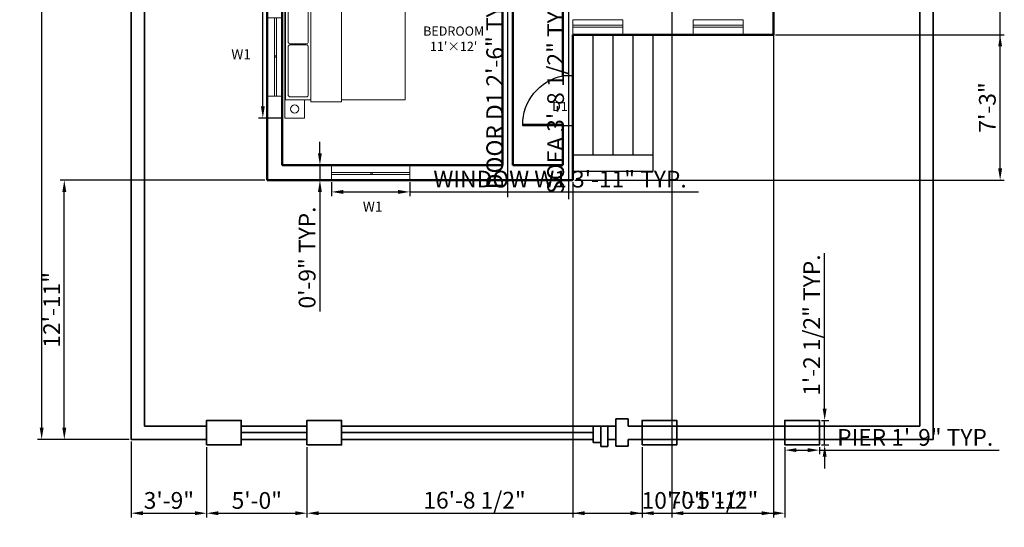
# Model space of a CAD drawing. Units: inches. Extents: x 452 to 1041, y 578 to 1412.
# Tile 1 of 3: x 452 to 1041, y 578 to 881. Entities that reach past the tile are written whole.
import ezdxf

# ---------------------------------------------------------------- set-up
doc = ezdxf.new("R2010")
doc.units = ezdxf.units.IN
doc.linetypes.add('ACAD_ISO03W100', pattern=[30, 12, -18])
doc.layers.get('Defpoints').update_dxf_attribs({"linetype": 'ACAD_ISO03W100'})
for name, color, linetype, lineweight in [('A-ANNO-DIMS', 2, 'Continuous', 18), ('A-ANNO-TEXT', 7, 'Continuous', 18), ('A-AREA-IDEN', 7, 'Continuous', 25), ('A-DOOR', 3, 'Continuous', 25), ('A-FLOR-STRS', 7, 'Continuous', 25), ('A-FURN', 8, 'Continuous', 18), ('A-GLAZ', 160, 'Continuous', 20), ('A-WALL', 7, 'Continuous', 50), ('C-PROP', 7, 'Continuous', 35)]:
    doc.layers.add(name, color=color, linetype=linetype, lineweight=lineweight)
doc.styles.get("Standard").update_dxf_attribs({"font": 'times.ttf'})
doc.dimstyles.new('ISO-25', dxfattribs={"dimscale": 2, "dimtxt": 5, "dimasz": 3.5, "dimexe": 1.25, "dimexo": 0.625, "dimtad": 1, "dimdsep": 46, "dimlunit": 3, "dimtxsty": 'Standard', "dimcen": 2.5, "dimadec": 0, "dimazin": 0, "dimtfac": 1, "dimtmove": 0, "dimatfit": 3, "dimfxl": 1, "dimarcsym": 0})

# ---------------------------------------------------------------- blocks, each defined once
blk = doc.blocks.new('D1')
for p, q in [((734.6, 1191.77), (733.6, 1191.77)), ((733.6, 1191.77), (733.6, 1167.77)), ((734.6, 1161.77), (734.6, 1191.77)), ((704.6, 1161.77), (704.6, 1167.77))]:
    blk.add_line(p, q)
blk.add_arc((733.85, 1161.94), 29.82, 89.51971, 168.74109)
blk = doc.blocks.new('W')
for p, q in [((913.24, 916.29), (913.24, 963.09)), ((913.24, 963.09), (922.24, 963.09)), ((917.74, 963.09), (917.74, 916.29)), ((918.94, 963.09), (918.94, 916.29)), ((922.24, 963.09), (922.24, 916.29)), ((917.74, 940.48), (918.94, 940.48)), ((917.74, 939.69), (918.94, 939.69)), ((922.24, 916.29), (913.24, 916.29))]:
    blk.add_line(p, q)
blk = doc.blocks.new('V')
for p, q in [((599.59, 961.66), (599.59, 991.66)), ((599.59, 991.66), (608.59, 991.66)), ((604.09, 961.66), (604.09, 991.66)), ((604.09, 991.66), (605.29, 991.66)), ((605.29, 991.66), (605.29, 961.66)), ((608.59, 991.66), (608.59, 961.66)), ((608.59, 961.66), (599.59, 961.66)), ((608.59, 961.66), (604.09, 961.66))]:
    blk.add_line(p, q)
blk = doc.blocks.new('*D8')
at = {"layer": 'A-ANNO-DIMS', "color": 0, "lineweight": -2, "transparency": 16777216}
for p, q in [((481.13, 1350.33), (462.24, 1350.33)), ((464.74, 1343.33), (464.74, 637.33)), ((481.13, 630.33), (462.24, 630.33))]:
    blk.add_line(p, q, dxfattribs=at)
at = {"layer": 'A-ANNO-DIMS', "color": 0, "lineweight": 70, "transparency": 16777216}
for points in [[(463.58, 1343.33), (465.91, 1343.33), (464.74, 1350.33)], [(463.58, 637.33), (465.91, 637.33), (464.74, 630.33)]]:
    blk.add_solid(points, dxfattribs=at)
at = {"layer": 'Defpoints', "color": 0, "lineweight": 70, "transparency": 16777216}
for p in [(482.38, 1350.33), (464.74, 630.33), (482.38, 630.33)]:
    blk.add_point(p, dxfattribs=at)
at = {"layer": 'A-ANNO-DIMS', "color": 0, "transparency": 16777216, "insert": (458.41, 990.33), "char_height": 10, "attachment_point": 5, "rotation": 90}
blk.add_mtext("60'", dxfattribs=at)
blk = doc.blocks.new('BED-FRAME-AND-SIDE-TABLES')
for p, q in [((0, 76.85), (15.53, 76.85)), ((0, 10.85), (0, 76.85)), ((0.5, 76.85), (0.5, 10.85)), ((33.97, 76.85), (72, 76.85)), ((72, 76.85), (72, 10.85)), ((15.53, 10.85), (0, 10.85)), ((72, 10.85), (33.97, 10.85))]:
    blk.add_line(p, q)
for points in [[(0, 76.85), (11.87, 76.85), (11.87, 87.71), (0, 87.71)], [(15.53, 78), (33.97, 78), (33.97, 9.68), (15.53, 9.68)], [(0, 0), (11.87, 0), (11.87, 10.85), (0, 10.85)]]:
    blk.add_lwpolyline(points, close=True)
for centre in [(5.89, 82.36), (5.89, 5.42)]:
    blk.add_circle(centre, 2.46)
blk = doc.blocks.new('BOUNDARY-PIER')
blk.add_lwpolyline([(0, 0), (20.76, 0), (20.76, 14.71), (0, 14.71)], close=True)
blk = doc.blocks.new('*D16')
at = {"layer": 'A-ANNO-DIMS', "color": 0, "lineweight": -2, "transparency": 16777216}
for p, q in [((638.26, 784.2), (638.26, 775.93)), ((685.06, 784.2), (685.06, 775.93)), ((645.26, 778.43), (678.06, 778.43)), ((685.06, 778.43), (857.83, 778.43))]:
    blk.add_line(p, q, dxfattribs=at)
at = {"layer": 'A-ANNO-DIMS', "color": 0, "lineweight": 70, "transparency": 16777216}
for points in [[(645.26, 779.6), (645.26, 777.26), (638.26, 778.43)], [(678.06, 779.6), (678.06, 777.26), (685.06, 778.43)]]:
    blk.add_solid(points, dxfattribs=at)
at = {"layer": 'Defpoints', "color": 0, "lineweight": 70, "transparency": 16777216}
for p in [(638.26, 785.45), (685.06, 785.45), (685.06, 778.43)]:
    blk.add_point(p, dxfattribs=at)
at = {"layer": 'A-ANNO-DIMS', "color": 0, "transparency": 16777216, "insert": (774.94, 784.79), "char_height": 10, "attachment_point": 5}
blk.add_mtext('WINDOW W1 3\'-11" TYP.', dxfattribs=at)
blk = doc.blocks.new('*D17')
at = {"layer": 'A-ANNO-DIMS', "color": 0, "lineweight": -2, "transparency": 16777216}
for p, q in [((631.24, 801.45), (631.24, 808.45)), ((637.01, 794.45), (628.74, 794.45)), ((631.24, 794.45), (631.24, 785.45)), ((637.01, 785.45), (628.74, 785.45)), ((631.24, 778.45), (631.24, 706.88))]:
    blk.add_line(p, q, dxfattribs=at)
at = {"layer": 'A-ANNO-DIMS', "color": 0, "lineweight": 70, "transparency": 16777216}
for points in [[(630.07, 801.45), (632.4, 801.45), (631.24, 794.45)], [(630.07, 778.45), (632.4, 778.45), (631.24, 785.45)]]:
    blk.add_solid(points, dxfattribs=at)
at = {"layer": 'Defpoints', "color": 0, "lineweight": 70, "transparency": 16777216}
for p in [(638.26, 794.45), (631.24, 785.45), (638.26, 785.45)]:
    blk.add_point(p, dxfattribs=at)
at = {"layer": 'A-ANNO-DIMS', "color": 0, "transparency": 16777216, "insert": (624.89, 739.17), "char_height": 10, "attachment_point": 5, "rotation": 90}
blk.add_mtext('0\'-9" TYP.', dxfattribs=at)
blk = doc.blocks.new('*D22')
at = {"layer": 'A-ANNO-DIMS', "color": 0, "lineweight": -2, "transparency": 16777216}
for p, q in [((740.23, 944.45), (746, 944.45)), ((743.5, 937.45), (743.5, 921.33)), ((740.23, 914.33), (746, 914.33)), ((743.5, 914.33), (743.5, 775.21))]:
    blk.add_line(p, q, dxfattribs=at)
at = {"layer": 'A-ANNO-DIMS', "color": 0, "lineweight": 70, "transparency": 16777216}
for points in [[(742.34, 937.45), (744.67, 937.45), (743.5, 944.45)], [(742.34, 921.33), (744.67, 921.33), (743.5, 914.33)]]:
    blk.add_solid(points, dxfattribs=at)
at = {"layer": 'Defpoints', "color": 0, "lineweight": 70, "transparency": 16777216}
for p in [(738.98, 944.45), (738.98, 914.33), (743.5, 914.33)]:
    blk.add_point(p, dxfattribs=at)
at = {"layer": 'A-ANNO-DIMS', "color": 0, "transparency": 16777216, "insert": (737.14, 841.27), "char_height": 10, "attachment_point": 5, "rotation": 90}
blk.add_mtext('DOOR D1 2\'-6" TYP.', dxfattribs=at)
blk = doc.blocks.new('*D26')
at = {"layer": 'A-ANNO-DIMS', "color": 0, "lineweight": -2, "transparency": 16777216}
for p, q in [((909.42, 625.82), (909.42, 621.45)), ((930.18, 625.82), (930.18, 621.45)), ((916.42, 623.95), (923.18, 623.95)), ((930.18, 623.95), (1037.72, 623.95))]:
    blk.add_line(p, q, dxfattribs=at)
at = {"layer": 'A-ANNO-DIMS', "color": 0, "lineweight": 70, "transparency": 16777216}
for points in [[(916.42, 625.12), (916.42, 622.79), (909.42, 623.95)], [(923.18, 625.12), (923.18, 622.79), (930.18, 623.95)]]:
    blk.add_solid(points, dxfattribs=at)
at = {"layer": 'Defpoints', "color": 0, "lineweight": 70, "transparency": 16777216}
for p in [(909.42, 627.07), (930.18, 627.07), (930.18, 623.95)]:
    blk.add_point(p, dxfattribs=at)
at = {"layer": 'A-ANNO-DIMS', "color": 0, "transparency": 16777216, "insert": (987.45, 630.3), "char_height": 10, "attachment_point": 5}
blk.add_mtext('PIER 1\'-9" TYP.', dxfattribs=at)
blk = doc.blocks.new('*D27')
at = {"layer": 'A-ANNO-DIMS', "color": 0, "lineweight": -2, "transparency": 16777216}
for p, q in [((933.29, 648.78), (933.29, 741.71)), ((931.43, 641.78), (935.79, 641.78)), ((933.29, 627.07), (933.29, 641.78)), ((931.43, 627.07), (935.79, 627.07)), ((933.29, 620.07), (933.29, 613.07))]:
    blk.add_line(p, q, dxfattribs=at)
at = {"layer": 'A-ANNO-DIMS', "color": 0, "lineweight": 70, "transparency": 16777216}
for points in [[(932.12, 648.78), (934.46, 648.78), (933.29, 641.78)], [(932.12, 620.07), (934.46, 620.07), (933.29, 627.07)]]:
    blk.add_solid(points, dxfattribs=at)
at = {"layer": 'Defpoints', "color": 0, "lineweight": 70, "transparency": 16777216}
for p in [(930.18, 641.78), (933.29, 641.78), (930.18, 627.07)]:
    blk.add_point(p, dxfattribs=at)
at = {"layer": 'A-ANNO-DIMS', "color": 0, "transparency": 16777216, "insert": (926.81, 698.75), "char_height": 10, "attachment_point": 5, "rotation": 90}
blk.add_mtext('1\'-2 1/2" TYP.', dxfattribs=at)
blk = doc.blocks.new('*D32')
at = {"layer": 'A-ANNO-DIMS', "color": 0, "lineweight": -2, "transparency": 16777216}
for p, q in [((785.53, 953.88), (777.57, 953.88)), ((780.07, 946.88), (780.07, 916.19)), ((785.53, 909.19), (777.57, 909.19)), ((780.07, 909.19), (780.07, 774.01))]:
    blk.add_line(p, q, dxfattribs=at)
at = {"layer": 'A-ANNO-DIMS', "color": 0, "lineweight": 70, "transparency": 16777216}
for points in [[(778.91, 946.88), (781.24, 946.88), (780.07, 953.88)], [(778.91, 916.19), (781.24, 916.19), (780.07, 909.19)]]:
    blk.add_solid(points, dxfattribs=at)
at = {"layer": 'Defpoints', "color": 0, "lineweight": 70, "transparency": 16777216}
for p in [(786.78, 953.88), (780.07, 909.19), (786.78, 909.19)]:
    blk.add_point(p, dxfattribs=at)
at = {"layer": 'A-ANNO-DIMS', "color": 0, "transparency": 16777216, "insert": (773.59, 838.1), "char_height": 10, "attachment_point": 5, "rotation": 90}
blk.add_mtext('SOFA 3\'-8 1/2" TYP.', dxfattribs=at)
blk = doc.blocks.new('*D34')
at = {"layer": 'A-ANNO-DIMS', "color": 0, "lineweight": -2, "transparency": 16777216}
for p, q in [((597.08, 910.3), (597.08, 1067.89)), ((608.99, 910.3), (594.58, 910.3)), ((597.08, 829.6), (597.08, 903.3)), ((608.99, 822.6), (594.58, 822.6))]:
    blk.add_line(p, q, dxfattribs=at)
at = {"layer": 'A-ANNO-DIMS', "color": 0, "lineweight": 70, "transparency": 16777216}
for points in [[(595.92, 903.3), (598.25, 903.3), (597.08, 910.3)], [(595.92, 829.6), (598.25, 829.6), (597.08, 822.6)]]:
    blk.add_solid(points, dxfattribs=at)
at = {"layer": 'Defpoints', "color": 0, "lineweight": 70, "transparency": 16777216}
for p in [(597.08, 910.3), (610.24, 910.3), (610.24, 822.6)]:
    blk.add_point(p, dxfattribs=at)
at = {"layer": 'A-ANNO-DIMS', "color": 0, "transparency": 16777216, "insert": (590.59, 992.6), "char_height": 10, "attachment_point": 5, "rotation": 90}
blk.add_mtext('BED SET 7\'-3 1/2" TYP.', dxfattribs=at)
blk = doc.blocks.new('*D39')
at = {"layer": 'A-ANNO-DIMS', "color": 0, "lineweight": -2, "transparency": 16777216}
for p, q in [((912.84, 1253.45), (1040.79, 1253.45)), ((1038.29, 792.45), (1038.29, 1246.45)), ((783.84, 785.45), (1040.79, 785.45))]:
    blk.add_line(p, q, dxfattribs=at)
at = {"layer": 'A-ANNO-DIMS', "color": 0, "lineweight": 70, "transparency": 16777216}
for points in [[(1037.13, 1246.45), (1039.46, 1246.45), (1038.29, 1253.45)], [(1037.13, 792.45), (1039.46, 792.45), (1038.29, 785.45)]]:
    blk.add_solid(points, dxfattribs=at)
at = {"layer": 'Defpoints', "color": 0, "lineweight": 70, "transparency": 16777216}
for p in [(911.59, 1253.45), (1038.29, 1253.45), (782.59, 785.45)]:
    blk.add_point(p, dxfattribs=at)
at = {"layer": 'A-ANNO-DIMS', "color": 0, "transparency": 16777216, "insert": (1031.94, 1019.45), "char_height": 10, "attachment_point": 5, "rotation": 90}
blk.add_mtext('39\'-0"', dxfattribs=at)
blk = doc.blocks.new('*D41')
at = {"layer": 'A-ANNO-DIMS', "color": 0, "lineweight": -2, "transparency": 16777216}
for p, q in [((598.34, 785.45), (475.79, 785.45)), ((478.29, 637.33), (478.29, 778.45)), ((517.04, 630.33), (475.79, 630.33))]:
    blk.add_line(p, q, dxfattribs=at)
at = {"layer": 'A-ANNO-DIMS', "color": 0, "lineweight": 70, "transparency": 16777216}
for points in [[(477.13, 778.45), (479.46, 778.45), (478.29, 785.45)], [(477.13, 637.33), (479.46, 637.33), (478.29, 630.33)]]:
    blk.add_solid(points, dxfattribs=at)
at = {"layer": 'Defpoints', "color": 0, "lineweight": 70, "transparency": 16777216}
for p in [(478.29, 785.45), (599.59, 785.45), (518.29, 630.33)]:
    blk.add_point(p, dxfattribs=at)
at = {"layer": 'A-ANNO-DIMS', "color": 0, "transparency": 16777216, "insert": (472.04, 707.89), "char_height": 10, "attachment_point": 5, "rotation": 90}
blk.add_mtext('12\'-11"', dxfattribs=at)
blk = doc.blocks.new('*D42')
at = {"layer": 'A-ANNO-DIMS', "color": 0, "lineweight": -2, "transparency": 16777216}
for p, q in [((518.29, 629.08), (518.29, 583.73)), ((563.46, 625.82), (563.46, 583.73)), ((525.29, 586.23), (556.46, 586.23))]:
    blk.add_line(p, q, dxfattribs=at)
at = {"layer": 'A-ANNO-DIMS', "color": 0, "lineweight": 70, "transparency": 16777216}
for points in [[(525.29, 587.4), (525.29, 585.07), (518.29, 586.23)], [(556.46, 587.4), (556.46, 585.07), (563.46, 586.23)]]:
    blk.add_solid(points, dxfattribs=at)
at = {"layer": 'Defpoints', "color": 0, "lineweight": 70, "transparency": 16777216}
for p in [(518.29, 630.33), (563.46, 627.07), (563.46, 586.23)]:
    blk.add_point(p, dxfattribs=at)
at = {"layer": 'A-ANNO-DIMS', "color": 0, "transparency": 16777216, "insert": (540.88, 592.59), "char_height": 10, "attachment_point": 5}
blk.add_mtext('3\'-9"', dxfattribs=at)
blk = doc.blocks.new('*D43')
at = {"layer": 'A-ANNO-DIMS', "color": 0, "lineweight": -2, "transparency": 16777216}
for p, q in [((563.46, 625.82), (563.46, 583.73)), ((623.5, 625.82), (623.5, 583.73)), ((570.46, 586.23), (616.5, 586.23))]:
    blk.add_line(p, q, dxfattribs=at)
at = {"layer": 'A-ANNO-DIMS', "color": 0, "lineweight": 70, "transparency": 16777216}
for points in [[(570.46, 587.4), (570.46, 585.07), (563.46, 586.23)], [(616.5, 587.4), (616.5, 585.07), (623.5, 586.23)]]:
    blk.add_solid(points, dxfattribs=at)
at = {"layer": 'Defpoints', "color": 0, "lineweight": 70, "transparency": 16777216}
for p in [(563.46, 627.07), (623.5, 627.07), (623.5, 586.23)]:
    blk.add_point(p, dxfattribs=at)
at = {"layer": 'A-ANNO-DIMS', "color": 0, "transparency": 16777216, "insert": (593.48, 592.57), "char_height": 10, "attachment_point": 5}
blk.add_mtext('5\'-0"', dxfattribs=at)
blk = doc.blocks.new('*D44')
at = {"layer": 'A-ANNO-DIMS', "color": 0, "lineweight": -2, "transparency": 16777216}
for p, q in [((623.5, 625.82), (623.5, 583.73)), ((824.04, 625.82), (824.04, 583.73)), ((630.5, 586.23), (817.04, 586.23))]:
    blk.add_line(p, q, dxfattribs=at)
at = {"layer": 'A-ANNO-DIMS', "color": 0, "lineweight": 70, "transparency": 16777216}
for points in [[(630.5, 587.4), (630.5, 585.07), (623.5, 586.23)], [(817.04, 587.4), (817.04, 585.07), (824.04, 586.23)]]:
    blk.add_solid(points, dxfattribs=at)
at = {"layer": 'Defpoints', "color": 0, "lineweight": 70, "transparency": 16777216}
for p in [(623.5, 627.07), (824.04, 627.07), (824.04, 586.23)]:
    blk.add_point(p, dxfattribs=at)
at = {"layer": 'A-ANNO-DIMS', "color": 0, "transparency": 16777216, "insert": (723.77, 592.71), "char_height": 10, "attachment_point": 5}
blk.add_mtext('16\'-8 1/2"', dxfattribs=at)
blk = doc.blocks.new('*D45')
at = {"layer": 'A-ANNO-DIMS', "color": 0, "lineweight": -2, "transparency": 16777216}
for p, q in [((824.04, 625.82), (824.04, 583.73)), ((909.42, 625.82), (909.42, 583.73)), ((831.04, 586.23), (902.42, 586.23))]:
    blk.add_line(p, q, dxfattribs=at)
at = {"layer": 'A-ANNO-DIMS', "color": 0, "lineweight": 70, "transparency": 16777216}
for points in [[(831.04, 587.4), (831.04, 585.07), (824.04, 586.23)], [(902.42, 587.4), (902.42, 585.07), (909.42, 586.23)]]:
    blk.add_solid(points, dxfattribs=at)
at = {"layer": 'Defpoints', "color": 0, "lineweight": 70, "transparency": 16777216}
for p in [(824.04, 627.07), (909.42, 627.07), (909.42, 586.23)]:
    blk.add_point(p, dxfattribs=at)
at = {"layer": 'A-ANNO-DIMS', "color": 0, "transparency": 16777216, "insert": (866.73, 592.71), "char_height": 10, "attachment_point": 5}
blk.add_mtext('7\'-1 1/2"', dxfattribs=at)
blk = doc.blocks.new('*D46')
at = {"layer": 'A-ANNO-DIMS', "color": 0, "lineweight": -2, "transparency": 16777216}
for p, q in [((902.59, 871.2), (902.59, 583.73)), ((782.59, 784.2), (782.59, 583.73)), ((789.59, 586.23), (895.59, 586.23))]:
    blk.add_line(p, q, dxfattribs=at)
at = {"layer": 'A-ANNO-DIMS', "color": 0, "lineweight": 70, "transparency": 16777216}
for points in [[(789.59, 587.4), (789.59, 585.07), (782.59, 586.23)], [(895.59, 587.4), (895.59, 585.07), (902.59, 586.23)]]:
    blk.add_solid(points, dxfattribs=at)
at = {"layer": 'Defpoints', "color": 0, "lineweight": 70, "transparency": 16777216}
for p in [(902.59, 872.45), (782.59, 785.45), (902.59, 586.23)]:
    blk.add_point(p, dxfattribs=at)
at = {"layer": 'A-ANNO-DIMS', "color": 0, "transparency": 16777216, "insert": (842.59, 592.57), "char_height": 10, "attachment_point": 5}
blk.add_mtext('10\'-0"', dxfattribs=at)
blk = doc.blocks.new('*D47')
at = {"layer": 'A-ANNO-DIMS', "color": 0, "lineweight": -2, "transparency": 16777216}
for p, q in [((903.84, 872.45), (1040.79, 872.45)), ((1038.29, 792.45), (1038.29, 865.45)), ((783.84, 785.45), (1040.79, 785.45))]:
    blk.add_line(p, q, dxfattribs=at)
at = {"layer": 'A-ANNO-DIMS', "color": 0, "lineweight": 70, "transparency": 16777216}
for points in [[(1037.13, 865.45), (1039.46, 865.45), (1038.29, 872.45)], [(1037.13, 792.45), (1039.46, 792.45), (1038.29, 785.45)]]:
    blk.add_solid(points, dxfattribs=at)
at = {"layer": 'Defpoints', "color": 0, "lineweight": 70, "transparency": 16777216}
for p in [(902.59, 872.45), (1038.29, 872.45), (782.59, 785.45)]:
    blk.add_point(p, dxfattribs=at)
at = {"layer": 'A-ANNO-DIMS', "color": 0, "transparency": 16777216, "insert": (1031.94, 828.95), "char_height": 10, "attachment_point": 5, "rotation": 90}
blk.add_mtext('7\'-3"', dxfattribs=at)
blk = doc.blocks.new('*D48')
at = {"layer": 'A-ANNO-DIMS', "color": 0, "lineweight": -2, "transparency": 16777216}
for p, q in [((841.74, 1219.2), (841.74, 583.73)), ((902.59, 1219.2), (902.59, 583.73)), ((848.74, 586.23), (895.59, 586.23))]:
    blk.add_line(p, q, dxfattribs=at)
at = {"layer": 'A-ANNO-DIMS', "color": 0, "lineweight": 70, "transparency": 16777216}
for points in [[(848.74, 587.4), (848.74, 585.07), (841.74, 586.23)], [(895.59, 587.4), (895.59, 585.07), (902.59, 586.23)]]:
    blk.add_solid(points, dxfattribs=at)
at = {"layer": 'Defpoints', "color": 0, "lineweight": 70, "transparency": 16777216}
for p in [(841.74, 1220.45), (902.59, 1220.45), (902.59, 586.23)]:
    blk.add_point(p, dxfattribs=at)
at = {"layer": 'A-ANNO-DIMS', "color": 0, "transparency": 16777216, "insert": (872.17, 592.57), "char_height": 10, "attachment_point": 5}
blk.add_mtext('5\'-1"', dxfattribs=at)

msp = doc.modelspace()

# ---------------------------------------------------------------- linework, layer by layer
at = {"layer": 'A-FLOR-STRS'}
for p, q in [((794.593, 872.451), (794.593, 800.451)), ((806.593, 872.451), (806.593, 800.451)), ((830.593, 872.451), (818.593, 872.451)), ((818.593, 872.451), (818.593, 800.451)), ((830.593, 800.451), (830.593, 872.451)), ((830.593, 800.451), (782.593, 800.451)), ((782.593, 800.451), (782.593, 790.851)), ((830.593, 790.851), (830.593, 800.451)), ((782.593, 790.851), (830.593, 790.851))]:
    msp.add_line(p, q, dxfattribs=at)
at = {"layer": 'A-FURN'}
for points in [[(613.452, 867.109), (623.078, 867.109, 0.4142136), (624.278, 868.309), (624.278, 897.087, 0.4142136), (623.078, 898.287), (613.452, 898.287, 0.4142136), (612.252, 897.087), (612.252, 868.309, 0.4142136)], [(613.452, 835.273), (623.078, 835.273, 0.4142136), (624.278, 836.473), (624.278, 865.251, 0.4142136), (623.078, 866.451), (613.452, 866.451, 0.4142136), (612.252, 865.251), (612.252, 836.473, 0.4142136)]]:
    msp.add_lwpolyline(points, format="xyb", close=True, dxfattribs=at)
at = {"layer": 'A-WALL'}
for p, q in [((776.593, 847.904), (776.593, 1013.451)), ((902.593, 1013.451), (902.593, 872.451)), ((746.593, 944.451), (746.593, 794.451)), ((599.593, 785.451), (599.593, 938.451)), ((608.593, 938.451), (608.593, 794.451)), ((740.593, 794.451), (740.593, 938.451)), ((782.593, 785.451), (782.593, 872.451)), ((902.593, 872.451), (782.593, 872.451)), ((776.593, 794.451), (776.593, 818.904)), ((608.593, 794.451), (740.593, 794.451)), ((746.593, 794.451), (776.593, 794.451)), ((608.593, 785.451), (599.593, 785.451)), ((746.593, 785.451), (608.593, 785.451)), ((746.593, 785.451), (782.593, 785.451))]:
    msp.add_line(p, q, dxfattribs=at)
at = {"layer": 'C-PROP'}
for p, q in [((518.294, 630.334), (518.294, 1350.334)), ((998.294, 1350.334), (998.294, 630.334)), ((526.294, 638.334), (526.294, 1342.334)), ((990.294, 1342.334), (990.294, 638.334)), ((815.747, 642.699), (808.425, 642.699)), ((808.425, 642.699), (808.425, 626.412)), ((815.747, 638.334), (815.747, 642.699)), ((563.463, 638.334), (526.294, 638.334)), ((623.499, 638.334), (584.225, 638.334)), ((808.425, 638.334), (644.26, 638.334)), ((799.428, 638.334), (794.711, 638.334)), ((794.711, 638.334), (794.711, 628.453)), ((799.428, 626.234), (799.428, 638.334)), ((808.425, 638.334), (803.59, 638.334)), ((803.59, 638.334), (803.59, 630.334)), ((990.294, 638.334), (815.747, 638.334)), ((824.04, 638.334), (815.747, 638.334)), ((584.225, 634.423), (623.499, 634.423)), ((644.26, 634.423), (794.711, 634.423)), ((563.463, 630.334), (518.294, 630.334)), ((623.499, 630.334), (584.225, 630.334)), ((794.711, 630.334), (644.26, 630.334)), ((794.711, 628.453), (799.428, 628.453)), ((803.59, 626.234), (799.428, 626.234)), ((803.59, 630.334), (808.425, 630.334)), ((803.59, 630.334), (803.59, 626.234)), ((808.425, 630.334), (803.59, 630.334)), ((808.425, 626.412), (815.747, 626.412)), ((998.294, 630.334), (815.747, 630.334)), ((815.747, 626.412), (815.747, 630.334)), ((815.747, 630.334), (824.04, 630.334))]:
    msp.add_line(p, q, dxfattribs=at)

# ---------------------------------------------------------------- block references
at = {"layer": 'A-DOOR', "xscale": -1, "rotation": 90}
msp.add_blockref('D1', (1944.36, 1552.503), dxfattribs=at)
at = {"layer": 'A-FURN'}
msp.add_blockref('BED-FRAME-AND-SIDE-TABLES', (610.239, 822.597), dxfattribs=at)
at = {"layer": 'A-GLAZ'}
msp.add_blockref('W', (-313.65, -80.554), dxfattribs=at)
for name, p, rotation in [('V', (1774.197, 272.857), 90), ('V', (1846.252, 272.857), 90), ('W', (-278.03, 1707.694), 270)]:
    msp.add_blockref(name, p, dxfattribs=dict(at, rotation=rotation))
at = {"layer": 'C-PROP'}
for p in [(563.463, 627.067), (623.498, 627.067), (824.039, 627.067), (909.415, 627.067)]:
    msp.add_blockref('BOUNDARY-PIER', p, dxfattribs=at)

# ---------------------------------------------------------------- texts
at = {"layer": 'A-ANNO-TEXT', "attachment_point": 1}
for s, insert, char_height in [('W1', (578.234, 863.803), 6), ('D1', (770.24, 832.315), 5.5), ('W1', (656.938, 772.636), 6)]:
    msp.add_mtext_dynamic_manual_height_columns(s, width=337.44086, gutter_width=12.5, heights=[0], dxfattribs=dict(at, insert=insert, char_height=char_height))
at = {"layer": 'A-AREA-IDEN', "insert": (542.563, 877.395), "char_height": 5.5, "attachment_point": 1}
msp.add_mtext_dynamic_manual_height_columns("\\pxqc;BEDROOM\\P11'×12'", width=337.44086, gutter_width=12.5, heights=[0], dxfattribs=at)

# ---------------------------------------------------------------- dimensions: what is measured, and where the dimension line sits
at = {"layer": 'A-ANNO-DIMS'}
for base, p1, p2, override, picture, middle in [((464.745, 630.334), (482.382, 1350.334), (482.382, 630.334), {"dimclrd": 0, "dimclre": 0, "dimclrt": 0}, '*D8', (458.408, 990.334)), ((1038.294, 1253.451), (782.593, 785.451), (911.593, 1253.451), {"dimdec": 1, "dimlfac": 1, "dimrnd": 0, "dimzin": 1, "dimdsep": 46, "dimlunit": 4, "dimfrac": 2}, '*D39', (1031.943, 1019.451)), ((1038.294, 872.451), (782.593, 785.451), (902.593, 872.451), {"dimdec": 1, "dimlfac": 1, "dimrnd": 0, "dimzin": 1, "dimdsep": 46, "dimlunit": 4, "dimfrac": 2}, '*D47', (1031.943, 828.951)), ((478.294, 785.451), (518.294, 630.334), (599.593, 785.451), {"dimdec": 1, "dimlfac": 1, "dimrnd": 0, "dimzin": 1, "dimdsep": 46, "dimlunit": 4, "dimfrac": 2}, '*D41', (472.044, 707.892))]:
    dim = msp.add_linear_dim(base=base, p1=p1, p2=p2, angle=90, dimstyle='ISO-25', override=override, dxfattribs=at)
    dim.commit()
    dim.dimension.update_dxf_attribs({"geometry": picture, "text_midpoint": middle})
for base, p1, p2, picture, middle in [((902.593, 586.234), (841.739, 1220.451), (902.593, 1220.451), '*D48', (872.166, 592.571)), ((902.593, 586.234), (782.593, 785.451), (902.593, 872.451), '*D46', (842.593, 592.571)), ((563.463, 586.234), (518.294, 630.334), (563.463, 627.067), '*D42', (540.879, 592.585)), ((623.499, 586.234), (563.463, 627.067), (623.499, 627.067), '*D43', (593.481, 592.571)), ((824.04, 586.234), (623.499, 627.067), (824.04, 627.067), '*D44', (723.769, 592.711)), ((909.415, 586.234), (824.04, 627.067), (909.415, 627.067), '*D45', (866.727, 592.711))]:
    dim = msp.add_linear_dim(base=base, p1=p1, p2=p2, dimstyle='ISO-25', override={"dimdec": 1, "dimlfac": 1, "dimrnd": 0, "dimzin": 1, "dimdsep": 46, "dimlunit": 4, "dimfrac": 2}, dxfattribs=at)
    dim.commit()
    dim.dimension.update_dxf_attribs({"geometry": picture, "text_midpoint": middle})
for base, p1, p2, angle, text, picture, middle in [((597.082, 910.304), (610.239, 822.597), (610.239, 910.304), 90, 'BED SET <> TYP.', '*D34', (590.594, 992.595)), ((780.074, 909.191), (786.777, 953.88), (786.777, 909.191), 270, 'SOFA <> TYP.', '*D32', (773.586, 838.101)), ((743.502, 914.331), (738.984, 944.451), (738.984, 914.331), 270, 'DOOR D1 <> TYP.', '*D22', (737.14, 841.272)), ((631.237, 785.451), (638.257, 794.451), (638.257, 785.451), 270, '<> TYP.', '*D17', (624.886, 739.166)), ((933.291, 641.78), (930.177, 627.067), (930.177, 641.78), 90, '<> TYP.', '*D27', (926.814, 698.746))]:
    dim = msp.add_linear_dim(base=base, p1=p1, p2=p2, angle=angle, text=text, dimstyle='ISO-25', override={"dimdec": 1, "dimlfac": 1, "dimrnd": 0, "dimzin": 1, "dimdsep": 46, "dimlunit": 4, "dimfrac": 2}, dxfattribs=at)
    dim.commit()
    dim.dimension.update_dxf_attribs({"geometry": picture, "text_midpoint": middle})
for base, p1, p2, text, picture, middle in [((685.057, 778.431), (638.257, 785.451), (685.057, 785.451), 'WINDOW W1 <> TYP.', '*D16', (774.943, 784.792)), ((930.177, 623.953), (909.415, 627.067), (930.177, 627.067), 'PIER <> TYP.', '*D26', (987.45, 630.304))]:
    dim = msp.add_linear_dim(base=base, p1=p1, p2=p2, text=text, dimstyle='ISO-25', override={"dimdec": 1, "dimlfac": 1, "dimrnd": 0, "dimzin": 1, "dimdsep": 46, "dimlunit": 4, "dimfrac": 2}, dxfattribs=at)
    dim.commit()
    dim.dimension.update_dxf_attribs({"geometry": picture, "text_midpoint": middle})

doc.saveas('drawing.dxf')
